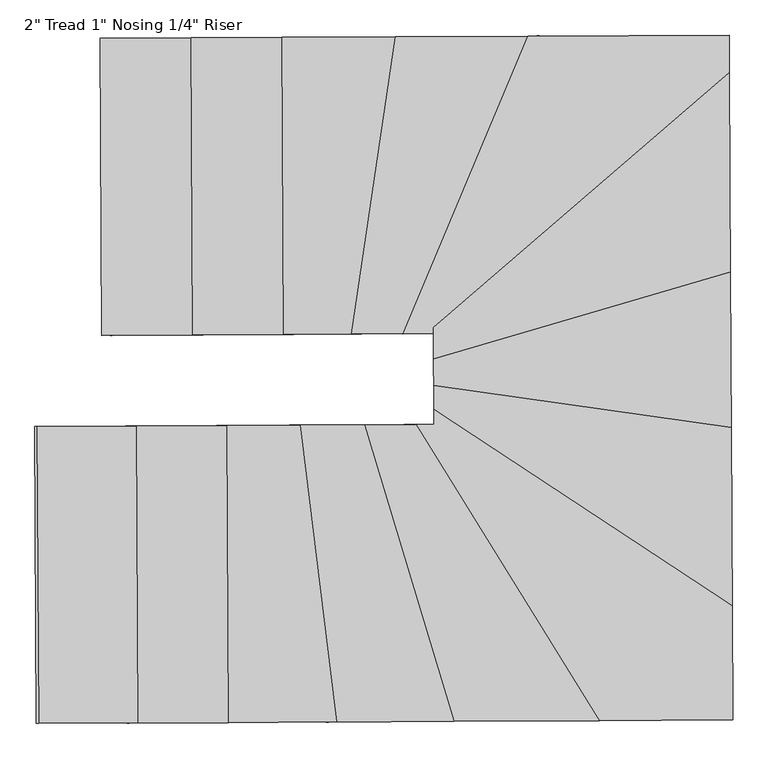
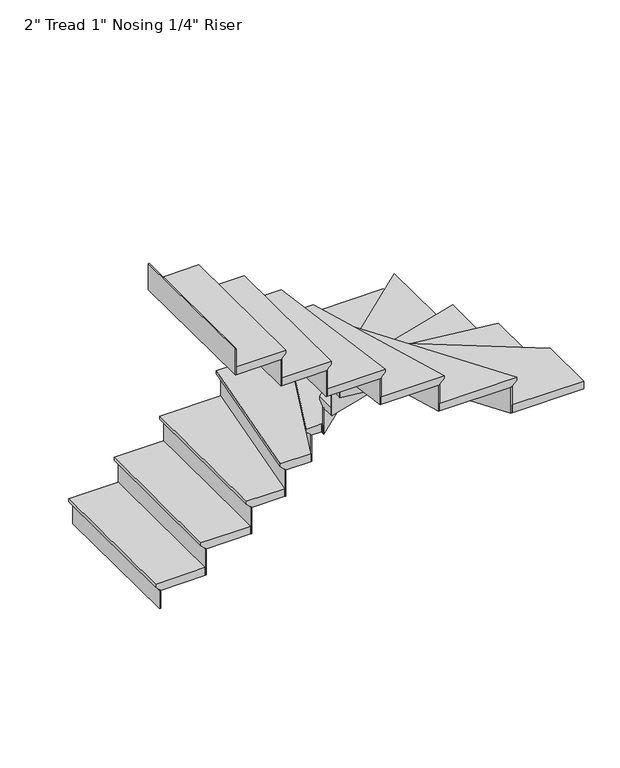
"""IFC4 building model written with IfcOpenShell, lengths in millimetres: stair flight geometry."""

from ifc_helpers import new_model, si_unit, origin, place, context, project, spatial, faceted_brep, source, transform, mapped, element, save


def stair_flight_0f4fe1b0(model_context):
    return source(origin(), model_context, "Body", "Brep", [
        faceted_brep([(73.5214139, -4197.1296428, 7059.0833333), (73.5214139, -4197.1296428, 7078.1333333), (68.8012135, -3282.7418259, 7078.1333333), (68.8012135, -3282.7418259, 7059.0833333), (98.9210755, -4196.9985261, 7033.6833333), (94.200875, -3282.6107092, 7033.6833333), (378.3173529, -4195.5562427, 7078.1333333), (373.5971524, -3281.1684258, 7078.1333333), (94.200875, -3282.6107092, 7027.3333333), (373.5971524, -3281.1684258, 7027.3333333), (378.3173529, -4195.5562427, 7027.3333333), (98.9210755, -4196.9985261, 7027.3333333)], [[[0, 1, 2, 3]], [[4, 0, 3, 5]], [[2, 1, 6, 7]], [[8, 9, 10, 11]], [[2, 7, 9, 8, 5, 3]], [[8, 11, 4, 5]], [[6, 1, 0, 4, 11, 10]], [[7, 6, 10, 9]]]),
        faceted_brep([(98.9210755, -4196.9985261, 7027.3333333), (98.9210755, -4196.9985261, 6908.8), (105.2709909, -4196.965747, 6908.8), (105.2709909, -4196.965747, 7027.3333333), (94.200875, -3282.6107092, 7027.3333333), (100.5507904, -3282.5779301, 7027.3333333), (100.5507904, -3282.5779301, 6908.8), (94.200875, -3282.6107092, 6908.8)], [[[0, 1, 2, 3]], [[4, 5, 6, 7]], [[1, 0, 4, 7]], [[2, 1, 7, 6]], [[3, 2, 6, 5]], [[0, 3, 5, 4]]]),
        faceted_brep([(378.3173529, -4195.5562427, 7196.6666667), (378.3173529, -4195.5562427, 7027.3333333), (384.6672683, -4195.5234635, 7027.3333333), (384.6672683, -4195.5234635, 7196.6666667), (373.5971524, -3281.1684258, 7196.6666667), (379.9470678, -3281.1356466, 7196.6666667), (379.9470678, -3281.1356466, 7027.3333333), (373.5971524, -3281.1684258, 7027.3333333)], [[[0, 1, 2, 3]], [[4, 5, 6, 7]], [[1, 0, 4, 7]], [[2, 1, 7, 6]], [[3, 2, 6, 5]], [[0, 3, 5, 4]]]),
        faceted_brep([(348.1974909, -3281.2995425, 7247.4666667), (352.9176913, -4195.6873594, 7247.4666667), (657.7136303, -4194.1139592, 7247.4666667), (652.9934298, -3279.7261423, 7247.4666667), (373.5971524, -3281.1684258, 7196.6666667), (652.9934298, -3279.7261423, 7196.6666667), (657.7136303, -4194.1139592, 7196.6666667), (378.3173529, -4195.5562427, 7196.6666667), (373.5971524, -3281.1684258, 7203.0166667), (348.1974909, -3281.2995425, 7228.4166667), (378.3173529, -4195.5562427, 7203.0166667), (352.9176913, -4195.6873594, 7228.4166667)], [[[0, 1, 2, 3]], [[4, 5, 6, 7]], [[0, 3, 5, 4, 8, 9]], [[4, 7, 10, 8]], [[2, 1, 11, 10, 7, 6]], [[3, 2, 6, 5]], [[11, 1, 0, 9]], [[10, 11, 9, 8]]]),
        faceted_brep([(657.7136303, -4194.1139592, 7366.0), (657.7136303, -4194.1139592, 7196.6666667), (664.0635457, -4194.08118, 7196.6666667), (664.0635457, -4194.08118, 7366.0), (652.9934298, -3279.7261423, 7366.0), (659.3433452, -3279.6933631, 7366.0), (659.3433452, -3279.6933631, 7196.6666667), (652.9934298, -3279.7261423, 7196.6666667)], [[[0, 1, 2, 3]], [[4, 5, 6, 7]], [[1, 0, 4, 7]], [[2, 1, 7, 6]], [[3, 2, 6, 5]], [[0, 3, 5, 4]]]),
        faceted_brep([(627.5937682, -3279.857259, 7416.8), (632.3139687, -4194.2450759, 7416.8), (866.9504995, -4193.0338486, 7416.8), (1003.1488336, -3277.9185901, 7416.8), (652.9934298, -3279.7261423, 7366.0), (1003.1488336, -3277.9185901, 7366.0), (866.9504995, -4193.0338486, 7366.0), (657.7136303, -4194.1139592, 7366.0), (652.9934298, -3279.7261423, 7372.35), (627.5937682, -3279.857259, 7397.75), (657.7136303, -4194.1139592, 7372.35), (632.3139687, -4194.2450759, 7397.75)], [[[0, 1, 2, 3]], [[4, 5, 6, 7]], [[0, 3, 5, 4, 8, 9]], [[4, 7, 10, 8]], [[2, 1, 11, 10, 7, 6]], [[3, 2, 6, 5]], [[11, 1, 0, 9]], [[10, 11, 9, 8]]]),
        faceted_brep([(866.9504995, -4193.0338486, 7535.3333333), (866.9504995, -4193.0338486, 7366.0), (873.3753797, -4193.0006825, 7366.0), (873.3753797, -4193.0006825, 7535.3333333), (1003.1488336, -3277.9185901, 7535.3333333), (1009.5737138, -3277.885424, 7535.3333333), (1009.5737138, -3277.885424, 7366.0), (1003.1488336, -3277.9185901, 7366.0)], [[[0, 1, 2, 3]], [[4, 5, 6, 7]], [[1, 0, 4, 7]], [[2, 1, 7, 6]], [[3, 2, 6, 5]], [[0, 3, 5, 4]]]),
        faceted_brep([(977.4493129, -3278.0512547, 7586.1333333), (841.2509788, -4193.1665132, 7586.1333333), (1028.3454494, -4192.2007049, 7586.1333333), (1412.7936505, -3275.8039451, 7586.1333333), (1003.1488336, -3277.9185901, 7535.3333333), (1412.7936505, -3275.8039451, 7535.3333333), (1028.3454494, -4192.2007049, 7535.3333333), (866.9504995, -4193.0338486, 7535.3333333), (1003.1488336, -3277.9185901, 7541.6833333), (977.4493129, -3278.0512547, 7567.0833333), (866.9504995, -4193.0338486, 7541.6833333), (841.2509788, -4193.1665132, 7567.0833333)], [[[0, 1, 2, 3]], [[4, 5, 6, 7]], [[0, 3, 5, 4, 8, 9]], [[4, 7, 10, 8]], [[2, 1, 11, 10, 7, 6]], [[3, 2, 6, 5]], [[11, 1, 0, 9]], [[10, 11, 9, 8]]]),
        faceted_brep([(1028.3454494, -4192.2007049, 7704.6666667), (1028.3454494, -4192.2007049, 7535.3333333), (1035.2465542, -4192.1650804, 7535.3333333), (1035.2465542, -4192.1650804, 7704.6666667), (1412.7936505, -3275.8039451, 7704.6666667), (1419.6947553, -3275.7683206, 7704.6666667), (1419.6947553, -3275.7683206, 7535.3333333), (1412.7936505, -3275.8039451, 7535.3333333)], [[[0, 1, 2, 3]], [[4, 5, 6, 7]], [[1, 0, 4, 7]], [[2, 1, 7, 6]], [[3, 2, 6, 5]], [[0, 3, 5, 4]]]),
        faceted_brep([(2004.5597861, -3422.5660243, 7755.4666667), (2003.7864306, -3272.753156, 7755.4666667), (1385.1892314, -3275.9464431, 7755.4666667), (1000.7410303, -4192.3432028, 7755.4666667), (1094.1188142, -4191.8611734, 7755.4666667), (1094.1970217, -4207.0113762, 7755.4666667), (2003.7864306, -3272.753156, 7704.6666667), (2004.5597861, -3422.5660243, 7704.6666667), (1094.1970217, -4207.0113762, 7704.6666667), (1094.1188142, -4191.8611734, 7704.6666667), (1028.3454494, -4192.2007049, 7704.6666667), (1412.7936505, -3275.8039451, 7704.6666667), (1028.3454494, -4192.2007049, 7711.0166667), (1412.7936505, -3275.8039451, 7711.0166667), (1000.7410303, -4192.3432028, 7736.4166667), (1385.1892314, -3275.9464431, 7736.4166667)], [[[0, 1, 2, 3, 4, 5]], [[6, 7, 8, 9, 10, 11]], [[1, 0, 7, 6]], [[11, 10, 12, 13]], [[4, 3, 14, 12, 10, 9]], [[0, 5, 8, 7]], [[14, 3, 2, 15]], [[12, 14, 15, 13]], [[2, 1, 6, 11, 13, 15]], [[5, 4, 9, 8]]]),
        faceted_brep([(1094.1970217, -4207.0113762, 7874.0), (1094.1970217, -4207.0113762, 7704.6666667), (1094.2401004, -4215.3564963, 7704.6666667), (1094.2401004, -4215.3564963, 7874.0), (2004.5597861, -3422.5660243, 7874.0), (2004.6028648, -3430.9111444, 7874.0), (2004.6028648, -3430.9111444, 7704.6666667), (2004.5597861, -3422.5660243, 7704.6666667)], [[[0, 1, 2, 3]], [[4, 5, 6, 7]], [[1, 0, 4, 7]], [[2, 1, 7, 6]], [[3, 2, 6, 5]], [[0, 3, 5, 4]]]),
        faceted_brep([(2004.3874713, -3389.1855438, 7924.8), (1094.0247069, -4173.6308957, 7924.8), (1094.654759, -4295.6833292, 7924.8), (2007.6910705, -4029.1522065, 7924.8), (2004.5597861, -3422.5660243, 7874.0), (2007.6910705, -4029.1522065, 7874.0), (1094.654759, -4295.6833292, 7874.0), (1094.1970217, -4207.0113762, 7874.0), (2004.5597861, -3422.5660243, 7880.35), (2004.3874713, -3389.1855438, 7905.75), (1094.1970217, -4207.0113762, 7880.35), (1094.0247069, -4173.6308957, 7905.75)], [[[0, 1, 2, 3]], [[4, 5, 6, 7]], [[0, 3, 5, 4, 8, 9]], [[4, 7, 10, 8]], [[3, 2, 6, 5]], [[11, 1, 0, 9]], [[10, 11, 9, 8]], [[2, 1, 11, 10, 7, 6]]]),
        faceted_brep([(1094.654759, -4295.6833292, 8043.3333333), (1094.654759, -4295.6833292, 7874.0), (1094.6888553, -4302.2884051, 7874.0), (1094.6888553, -4302.2884051, 8043.3333333), (2007.6910705, -4029.1522065, 8043.3333333), (2007.7251669, -4035.7572823, 8043.3333333), (2007.7251669, -4035.7572823, 7874.0), (2007.6910705, -4029.1522065, 7874.0)], [[[0, 1, 2, 3]], [[4, 5, 6, 7]], [[1, 0, 4, 7]], [[2, 1, 7, 6]], [[3, 2, 6, 5]], [[0, 3, 5, 4]]]),
        faceted_brep([(2007.5546851, -4002.7319029, 8094.1333333), (1094.5183736, -4269.2630257, 8094.1333333), (1095.0784269, -4377.7554326, 8094.1333333), (2010.1530082, -4506.0738629, 8094.1333333), (2007.6910705, -4029.1522065, 8043.3333333), (2010.1530082, -4506.0738629, 8043.3333333), (1095.0784269, -4377.7554326, 8043.3333333), (1094.654759, -4295.6833292, 8043.3333333), (2007.6910705, -4029.1522065, 8049.6833333), (2007.5546851, -4002.7319029, 8075.0833333), (1094.654759, -4295.6833292, 8049.6833333), (1094.5183736, -4269.2630257, 8075.0833333)], [[[0, 1, 2, 3]], [[4, 5, 6, 7]], [[0, 3, 5, 4, 8, 9]], [[4, 7, 10, 8]], [[2, 1, 11, 10, 7, 6]], [[3, 2, 6, 5]], [[11, 1, 0, 9]], [[10, 11, 9, 8]]]),
        faceted_brep([(1095.0784269, -4377.7554326, 8212.6666667), (1095.0784269, -4377.7554326, 8043.3333333), (1095.1115512, -4384.1722058, 8043.3333333), (1095.1115512, -4384.1722058, 8212.6666667), (2010.1530082, -4506.0738629, 8212.6666667), (2010.1861325, -4512.4906361, 8212.6666667), (2010.1861325, -4512.4906361, 8043.3333333), (2010.1530082, -4506.0738629, 8043.3333333)], [[[0, 1, 2, 3]], [[4, 5, 6, 7]], [[1, 0, 4, 7]], [[2, 1, 7, 6]], [[3, 2, 6, 5]], [[0, 3, 5, 4]]]),
        faceted_brep([(2010.020511, -4480.40677, 8263.4666667), (1094.9459297, -4352.0883397, 8263.4666667), (1095.4823291, -4455.9985745, 8263.4666667), (2013.0146854, -5060.4322638, 8263.4666667), (2010.1530082, -4506.0738629, 8212.6666667), (2013.0146854, -5060.4322638, 8212.6666667), (1095.4823291, -4455.9985745, 8212.6666667), (1095.0784269, -4377.7554326, 8212.6666667), (2010.1530082, -4506.0738629, 8219.0166667), (2010.020511, -4480.40677, 8244.4166667), (1095.0784269, -4377.7554326, 8219.0166667), (1094.9459297, -4352.0883397, 8244.4166667)], [[[0, 1, 2, 3]], [[4, 5, 6, 7]], [[0, 3, 5, 4, 8, 9]], [[4, 7, 10, 8]], [[3, 2, 6, 5]], [[11, 1, 0, 9]], [[10, 11, 9, 8]], [[2, 1, 11, 10, 7, 6]]]),
        faceted_brep([(1095.4823291, -4455.9985745, 8382.0), (1095.4823291, -4455.9985745, 8212.6666667), (1095.5217161, -4463.6285363, 8212.6666667), (1095.5217161, -4463.6285363, 8382.0), (2013.0146854, -5060.4322638, 8382.0), (2013.0540723, -5068.0622255, 8382.0), (2013.0540723, -5068.0622255, 8212.6666667), (2013.0146854, -5060.4322638, 8212.6666667)], [[[0, 1, 2, 3]], [[4, 5, 6, 7]], [[1, 0, 4, 7]], [[2, 1, 7, 6]], [[3, 2, 6, 5]], [[0, 3, 5, 4]]]),
        faceted_brep([(1574.7396622, -5383.1960459, 8432.8), (2014.669115, -5380.9250672, 8432.8), (2012.8571376, -5029.9124167, 8432.8), (1095.3247813, -4425.4787274, 8432.8), (1095.5610976, -4471.2574507, 8432.8), (1010.2079956, -4471.6980556, 8432.8), (2014.669115, -5380.9250672, 8382.0), (1574.7396622, -5383.1960459, 8382.0), (1010.2079956, -4471.6980556, 8382.0), (1095.5610976, -4471.2574507, 8382.0), (1095.4823291, -4455.9985745, 8382.0), (2013.0146854, -5060.4322638, 8382.0), (1095.4823291, -4455.9985745, 8388.35), (2013.0146854, -5060.4322638, 8388.35), (1095.3247813, -4425.4787274, 8413.75), (2012.8571376, -5029.9124167, 8413.75)], [[[0, 1, 2, 3, 4, 5]], [[6, 7, 8, 9, 10, 11]], [[1, 0, 7, 6]], [[11, 10, 12, 13]], [[4, 3, 14, 12, 10, 9]], [[0, 5, 8, 7]], [[14, 3, 2, 15]], [[12, 14, 15, 13]], [[5, 4, 9, 8]], [[2, 1, 6, 11, 13, 15]]]),
        faceted_brep([(1010.2079956, -4471.6980556, 8551.3333333), (1010.2079956, -4471.6980556, 8382.0), (1002.7625472, -4471.7364901, 8382.0), (1002.7625472, -4471.7364901, 8551.3333333), (1574.7396622, -5383.1960459, 8551.3333333), (1567.2942139, -5383.2344803, 8551.3333333), (1567.2942139, -5383.2344803, 8382.0), (1574.7396622, -5383.1960459, 8382.0)], [[[0, 1, 2, 3]], [[4, 5, 6, 7]], [[1, 0, 4, 7]], [[2, 1, 7, 6]], [[3, 2, 6, 5]], [[0, 3, 5, 4]]]),
        faceted_brep([(1604.5214555, -5383.042308, 8602.1333333), (1039.9897889, -4471.5443178, 8602.1333333), (854.9585932, -4472.4994752, 8602.1333333), (1130.3137603, -5385.4902358, 8602.1333333), (1574.7396622, -5383.1960459, 8551.3333333), (1130.3137603, -5385.4902358, 8551.3333333), (854.9585932, -4472.4994752, 8551.3333333), (1010.2079956, -4471.6980556, 8551.3333333), (1574.7396622, -5383.1960459, 8557.6833333), (1604.5214555, -5383.042308, 8583.0833333), (1010.2079956, -4471.6980556, 8557.6833333), (1039.9897889, -4471.5443178, 8583.0833333)], [[[0, 1, 2, 3]], [[4, 5, 6, 7]], [[0, 3, 5, 4, 8, 9]], [[4, 7, 10, 8]], [[2, 1, 11, 10, 7, 6]], [[3, 2, 6, 5]], [[11, 1, 0, 9]], [[10, 11, 9, 8]]]),
        faceted_brep([(854.9585932, -4472.4994752, 8720.6666667), (854.9585932, -4472.4994752, 8551.3333333), (848.3363877, -4472.53366, 8551.3333333), (848.3363877, -4472.53366, 8720.6666667), (1130.3137603, -5385.4902358, 8720.6666667), (1123.6915548, -5385.5244206, 8720.6666667), (1123.6915548, -5385.5244206, 8551.3333333), (1130.3137603, -5385.4902358, 8551.3333333)], [[[0, 1, 2, 3]], [[4, 5, 6, 7]], [[1, 0, 4, 7]], [[2, 1, 7, 6]], [[3, 2, 6, 5]], [[0, 3, 5, 4]]]),
        faceted_brep([(1156.8025822, -5385.3534967, 8771.4666667), (881.4474152, -4472.3627361, 8771.4666667), (657.851655, -4473.5169694, 8771.4666667), (770.454123, -5387.3478826, 8771.4666667), (1130.3137603, -5385.4902358, 8720.6666667), (770.454123, -5387.3478826, 8720.6666667), (657.851655, -4473.5169694, 8720.6666667), (854.9585932, -4472.4994752, 8720.6666667), (1130.3137603, -5385.4902358, 8727.0166667), (1156.8025822, -5385.3534967, 8752.4166667), (854.9585932, -4472.4994752, 8727.0166667), (881.4474152, -4472.3627361, 8752.4166667)], [[[0, 1, 2, 3]], [[4, 5, 6, 7]], [[0, 3, 5, 4, 8, 9]], [[4, 7, 10, 8]], [[2, 1, 11, 10, 7, 6]], [[3, 2, 6, 5]], [[11, 1, 0, 9]], [[10, 11, 9, 8]]]),
        faceted_brep([(657.851655, -4473.5169694, 8890.0), (657.851655, -4473.5169694, 8720.6666667), (651.457697, -4473.5499759, 8720.6666667), (651.457697, -4473.5499759, 8890.0), (770.454123, -5387.3478826, 8890.0), (764.060165, -5387.3808891, 8890.0), (764.060165, -5387.3808891, 8720.6666667), (770.454123, -5387.3478826, 8720.6666667)], [[[0, 1, 2, 3]], [[4, 5, 6, 7]], [[1, 0, 4, 7]], [[2, 1, 7, 6]], [[3, 2, 6, 5]], [[0, 3, 5, 4]]]),
        faceted_brep([(796.0299553, -5387.2158565, 8940.8), (683.4274873, -4473.3849433, 8940.8), (432.5726821, -4474.6798916, 8940.8), (437.2928826, -5389.0677085, 8940.8), (770.454123, -5387.3478826, 8890.0), (437.2928826, -5389.0677085, 8890.0), (432.5726821, -4474.6798916, 8890.0), (657.851655, -4473.5169694, 8890.0), (770.454123, -5387.3478826, 8896.35), (796.0299553, -5387.2158565, 8921.75), (657.851655, -4473.5169694, 8896.35), (683.4274873, -4473.3849433, 8921.75)], [[[0, 1, 2, 3]], [[4, 5, 6, 7]], [[0, 3, 5, 4, 8, 9]], [[4, 7, 10, 8]], [[2, 1, 11, 10, 7, 6]], [[3, 2, 6, 5]], [[11, 1, 0, 9]], [[10, 11, 9, 8]]]),
        faceted_brep([(432.5726821, -4474.6798916, 9059.3333333), (432.5726821, -4474.6798916, 8890.0), (426.2227667, -4474.7126708, 8890.0), (426.2227667, -4474.7126708, 9059.3333333), (437.2928826, -5389.0677085, 9059.3333333), (430.9429672, -5389.1004877, 9059.3333333), (430.9429672, -5389.1004877, 8890.0), (437.2928826, -5389.0677085, 8890.0)], [[[0, 1, 2, 3]], [[4, 5, 6, 7]], [[1, 0, 4, 7]], [[2, 1, 7, 6]], [[3, 2, 6, 5]], [[0, 3, 5, 4]]]),
        faceted_brep([(462.6925441, -5388.9365918, 9110.1333333), (457.9723437, -4474.5487749, 9110.1333333), (153.1764047, -4476.1221751, 9110.1333333), (157.8966052, -5390.509992, 9110.1333333), (437.2928826, -5389.0677085, 9059.3333333), (157.8966052, -5390.509992, 9059.3333333), (153.1764047, -4476.1221751, 9059.3333333), (432.5726821, -4474.6798916, 9059.3333333), (437.2928826, -5389.0677085, 9065.6833333), (462.6925441, -5388.9365918, 9091.0833333), (432.5726821, -4474.6798916, 9065.6833333), (457.9723437, -4474.5487749, 9091.0833333)], [[[0, 1, 2, 3]], [[4, 5, 6, 7]], [[0, 3, 5, 4, 8, 9]], [[4, 7, 10, 8]], [[2, 1, 11, 10, 7, 6]], [[3, 2, 6, 5]], [[11, 1, 0, 9]], [[10, 11, 9, 8]]]),
        faceted_brep([(153.1764047, -4476.1221751, 9228.6666667), (153.1764047, -4476.1221751, 9059.3333333), (146.8264893, -4476.1549542, 9059.3333333), (146.8264893, -4476.1549542, 9228.6666667), (157.8966052, -5390.509992, 9228.6666667), (151.5466898, -5390.5427711, 9228.6666667), (151.5466898, -5390.5427711, 9059.3333333), (157.8966052, -5390.509992, 9059.3333333)], [[[0, 1, 2, 3]], [[4, 5, 6, 7]], [[1, 0, 4, 7]], [[2, 1, 7, 6]], [[3, 2, 6, 5]], [[0, 3, 5, 4]]]),
        faceted_brep([(-126.2198726, -4477.5644585, 9398.0), (-126.2198726, -4477.5644585, 9228.6666667), (-132.569788, -4477.5972377, 9228.6666667), (-132.569788, -4477.5972377, 9398.0), (-121.4996722, -5391.9522754, 9398.0), (-127.8495876, -5391.9850546, 9398.0), (-127.8495876, -5391.9850546, 9228.6666667), (-121.4996722, -5391.9522754, 9228.6666667)], [[[0, 1, 2, 3]], [[4, 5, 6, 7]], [[1, 0, 4, 7]], [[2, 1, 7, 6]], [[3, 2, 6, 5]], [[0, 3, 5, 4]]]),
        faceted_brep([(183.2962668, -5390.3788753, 9279.4666667), (178.5760663, -4475.9910584, 9279.4666667), (-126.2198726, -4477.5644585, 9279.4666667), (-121.4996722, -5391.9522754, 9279.4666667), (157.8966052, -5390.509992, 9228.6666667), (-121.4996722, -5391.9522754, 9228.6666667), (-126.2198726, -4477.5644585, 9228.6666667), (153.1764047, -4476.1221751, 9228.6666667), (157.8966052, -5390.509992, 9235.0166667), (183.2962668, -5390.3788753, 9260.4166667), (153.1764047, -4476.1221751, 9235.0166667), (178.5760663, -4475.9910584, 9260.4166667)], [[[0, 1, 2, 3]], [[4, 5, 6, 7]], [[0, 3, 5, 4, 8, 9]], [[4, 7, 10, 8]], [[2, 1, 11, 10, 7, 6]], [[3, 2, 6, 5]], [[11, 1, 0, 9]], [[10, 11, 9, 8]]]),
    ])


if __name__ == "__main__":
    model = new_model("IFC4")
    model_context = context("Model", 3, world=origin())
    ifc_project = project(units=[si_unit("LENGTHUNIT", "METRE", prefix="MILLI")], contexts=[model_context])
    site = spatial("IfcSite", under=ifc_project)
    building = spatial("IfcBuilding", under=site)
    placement = place(None, origin())
    stair_flight_shape = stair_flight_0f4fe1b0(model_context)
    element("IfcStairFlight", 1, ObjectType="2\" Tread 1\" Nosing 1/4\" Riser", at=placement, inside=building, context=model_context, shape_type="MappedRepresentation", body=[
        mapped(stair_flight_shape, transform((0.0, 0.0, 0.0), x_axis=(1.0, 0.0, 0.0), y_axis=(0.0, 1.0, 0.0), z_axis=(0.0, 0.0, 1.0))),
    ])
    save(model, "model.ifc")
